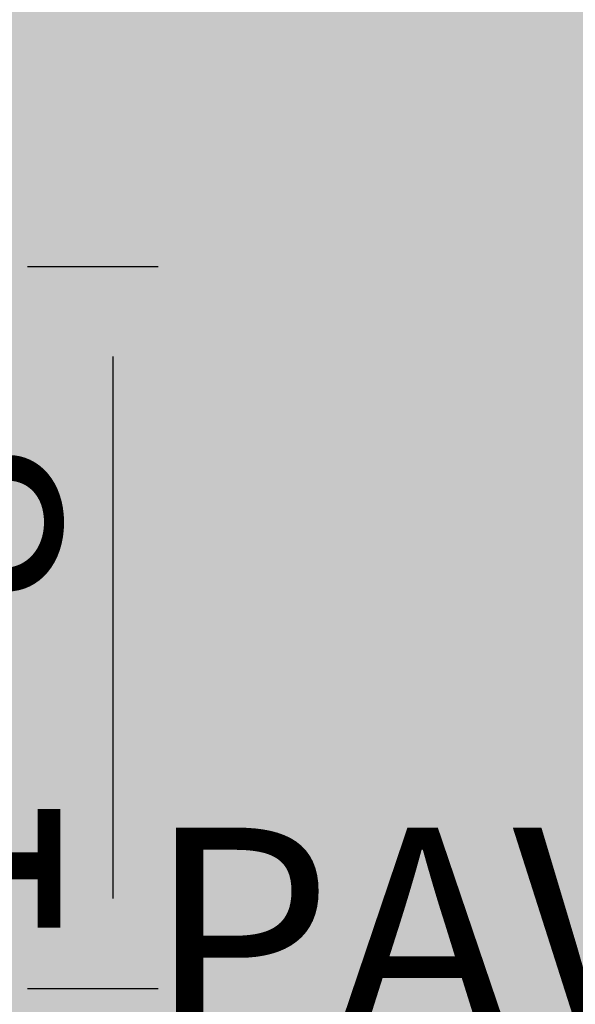
# Model space of a CAD drawing. Units: inches. Extents: x 459864 to 460310, y 324185 to 324787.
# Tile 55 of 112: x 460153 to 460169, y 324211 to 324239. Entities that reach past the tile are written whole.
import ezdxf

# ---------------------------------------------------------------- set-up
doc = ezdxf.new("R2010")
doc.units = ezdxf.units.IN
doc.layers.add('A-ANNO-DIMS', color=2, linetype='Continuous', lineweight=18)
doc.layers.add('L-SITE-PATT', color=252, linetype='Continuous', lineweight=13)
doc.styles.get("Standard").update_dxf_attribs({"font": 'arial.ttf'})
doc.dimstyles.new('ISO-25', dxfattribs={"dimtxt": 6, "dimasz": 2.5, "dimexe": 1.25, "dimexo": 0.625, "dimtad": 1, "dimdec": 1, "dimlunit": 3, "dimtxsty": 'Standard', "dimcen": 2.5, "dimadec": 0, "dimazin": 0, "dimtfac": 1, "dimtdec": 1, "dimtmove": 0, "dimatfit": 3, "dimfxl": 1, "dimarcsym": 0})

# ---------------------------------------------------------------- blocks, each defined once
blk = doc.blocks.new('*D34')
at = {"layer": 'A-ANNO-DIMS', "color": 0, "lineweight": -2, "transparency": 16777216}
for p, q in [((460132.814, 324211.063), (460132.814, 324207.434)), ((460152.838, 324211.063), (460152.838, 324207.434)), ((460135.314, 324208.684), (460150.338, 324208.684)), ((460152.838, 324208.684), (460202.984, 324208.684))]:
    blk.add_line(p, q, dxfattribs=at)
at = {"layer": 'A-ANNO-DIMS', "color": 0, "transparency": 16777216}
for points in [[(460135.314, 324209.101), (460135.314, 324208.268), (460132.814, 324208.684)], [(460150.338, 324209.101), (460150.338, 324208.268), (460152.838, 324208.684)]]:
    blk.add_solid(points, dxfattribs=at)
at = {"layer": 'Defpoints', "color": 0, "transparency": 16777216}
for p in [(460132.814, 324211.688), (460152.838, 324211.688), (460152.838, 324208.684)]:
    blk.add_point(p, dxfattribs=at)
at = {"layer": 'A-ANNO-DIMS', "color": 0, "transparency": 16777216, "insert": (460179.161, 324212.373), "char_height": 6, "attachment_point": 5}
blk.add_mtext('PAVER 1\'-8"', dxfattribs=at)
blk = doc.blocks.new('*D35')
at = {"layer": 'A-ANNO-DIMS', "color": 0, "lineweight": -2, "transparency": 16777216}
for p, q in [((460153.463, 324231.712), (460157.092, 324231.712)), ((460155.842, 324214.188), (460155.842, 324229.212)), ((460153.463, 324211.688), (460157.092, 324211.688))]:
    blk.add_line(p, q, dxfattribs=at)
at = {"layer": 'A-ANNO-DIMS', "color": 0, "transparency": 16777216}
for points in [[(460155.425, 324229.212), (460156.258, 324229.212), (460155.842, 324231.712)], [(460155.425, 324214.188), (460156.258, 324214.188), (460155.842, 324211.688)]]:
    blk.add_solid(points, dxfattribs=at)
at = {"layer": 'Defpoints', "color": 0, "transparency": 16777216}
for p in [(460152.838, 324231.712), (460155.842, 324231.712), (460152.838, 324211.688)]:
    blk.add_point(p, dxfattribs=at)
at = {"layer": 'A-ANNO-DIMS', "color": 0, "transparency": 16777216, "insert": (460152.153, 324221.7), "char_height": 6, "attachment_point": 5, "rotation": 90}
blk.add_mtext('1\'-8"', dxfattribs=at)

msp = doc.modelspace()

# ---------------------------------------------------------------- hatches: boundary and pattern name
at = {"layer": 'L-SITE-PATT'}
h = msp.add_hatch(dxfattribs=at)
h.set_pattern_fill('DOTS', color=256)
h.paths.add_polyline_path([(460269.804, 324283.483), (460247.115, 324283.483), (460121.929, 324283.483), (460121.929, 324252.473), (460117.429, 324252.473), (460110.124, 324252.473), (460110.124, 324243.287), (460080.83, 324243.287), (460080.83, 324252.473), (460061.115, 324252.473), (460061.115, 324251.882), (460077.909, 324251.882), (460077.909, 324199.483), (460080.83, 324199.483), (460080.83, 324207.553), (460110.124, 324207.553), (460110.124, 324199.483), (460110.813, 324199.483), (460262.115, 324199.483), (460269.804, 324199.483)], flags=17)
edge = h.paths.add_edge_path(flags=0)
edge.add_ellipse((460222.59, 324263.813), major_axis=(-8.485, 8.485), ratio=1, start_angle=405, end_angle=495, ccw=False)
edge.add_line((460214.821, 324254.66), (460214.832, 324254.666))
edge.add_ellipse((460222.59, 324263.813), major_axis=(-8.485, 8.485), ratio=1, start_angle=405, end_angle=495, ccw=False)
edge.add_line((460210.759, 324261.781), (460210.768, 324261.787))
edge.add_ellipse((460222.59, 324263.813), major_axis=(-8.485, 8.485), ratio=1, start_angle=405, end_angle=495, ccw=False)
edge.add_ellipse((460222.59, 324263.813), major_axis=(-8.485, 8.485), ratio=1, start_angle=392.754, end_angle=405, ccw=False)
edge.add_ellipse((460222.59, 324263.813), major_axis=(-8.485, 8.485), ratio=1, start_angle=380.9347, end_angle=392.754, ccw=False)
edge.add_line((460211.337, 324267.985), (460211.34, 324267.985))
edge.add_ellipse((460222.59, 324263.813), major_axis=(-8.485, 8.485), ratio=1, start_angle=380.9347, end_angle=392.754, ccw=False)
edge.add_ellipse((460222.59, 324263.813), major_axis=(-8.485, 8.485), ratio=1, start_angle=347.9015, end_angle=380.9347, ccw=False)
edge.add_ellipse((460222.59, 324263.813), major_axis=(-8.485, 8.485), ratio=1, start_angle=327.0619, end_angle=347.9015, ccw=False)
edge.add_ellipse((460222.59, 324263.813), major_axis=(-8.485, 8.485), ratio=1, start_angle=278.3246, end_angle=327.0619, ccw=False)
edge.add_line((460225.158, 324275.536), (460225.158, 324275.535))
edge.add_ellipse((460222.59, 324263.813), major_axis=(-8.485, 8.485), ratio=1, start_angle=278.3246, end_angle=327.0619, ccw=False)
edge.add_ellipse((460222.59, 324263.813), major_axis=(-8.485, 8.485), ratio=1, start_angle=260.6436, end_angle=278.3246, ccw=False)
edge.add_ellipse((460222.59, 324263.813), major_axis=(-8.485, 8.485), ratio=1, start_angle=225, end_angle=260.6436, ccw=False)
edge.add_line((460234.509, 324265.243), (460234.501, 324265.239))
edge.add_ellipse((460222.59, 324263.813), major_axis=(-8.485, 8.485), ratio=1, start_angle=225, end_angle=260.6436, ccw=False)
edge.add_ellipse((460222.59, 324263.813), major_axis=(-8.485, 8.485), ratio=1, start_angle=495, end_angle=585, ccw=False)
edge.add_line((460234.437, 324261.861), (460234.424, 324261.858))
edge.add_ellipse((460222.59, 324263.813), major_axis=(-8.485, 8.485), ratio=1, start_angle=495, end_angle=585, ccw=False)
edge.add_line((460227.95, 324253.067), (460227.946, 324253.083))
edge.add_ellipse((460222.59, 324263.813), major_axis=(-8.485, 8.485), ratio=1, start_angle=495, end_angle=585, ccw=False)
edge.add_line((460226.223, 324252.369), (460226.211, 324252.38))
edge.add_ellipse((460222.59, 324263.813), major_axis=(-8.485, 8.485), ratio=1, start_angle=495, end_angle=585, ccw=False)
h.paths.add_polyline_path([(460219.651, 324254.347), (460218.461, 324253.545), (460218.275, 324254.789), (460219.642, 324256.542), (460219.625, 324260.848), (460216.11, 324257.333), (460214.35, 324256.978), (460215.416, 324259.356), (460212.524, 324258.496), (460213.137, 324259.93), (460218.507, 324263.813), (460222.59, 324263.813), (460222.59, 324267.807), (460218.176, 324272.212), (460219.026, 324274.639), (460222.59, 324272.811), (460222.59, 324275.423), (460223.057, 324274.825), (460222.675, 324273.492), (460225.912, 324267.135), (460219.625, 324260.848)], flags=0)
edge = h.paths.add_edge_path(flags=0)
edge.add_ellipse((460194.576, 324264.046), major_axis=(-8.485, 8.485), ratio=1, start_angle=495, end_angle=585, ccw=False)
edge.add_line((460199.936, 324253.3), (460199.932, 324253.316))
edge.add_ellipse((460194.576, 324264.046), major_axis=(-8.485, 8.485), ratio=1, start_angle=495, end_angle=585, ccw=False)
edge.add_line((460198.208, 324252.603), (460198.196, 324252.613))
edge.add_ellipse((460194.576, 324264.046), major_axis=(-8.485, 8.485), ratio=1, start_angle=495, end_angle=585, ccw=False)
edge.add_ellipse((460194.576, 324264.046), major_axis=(-8.485, 8.485), ratio=1, start_angle=405, end_angle=495, ccw=False)
edge.add_line((460186.806, 324254.893), (460186.817, 324254.899))
edge.add_ellipse((460194.576, 324264.046), major_axis=(-8.485, 8.485), ratio=1, start_angle=405, end_angle=495, ccw=False)
edge.add_line((460182.744, 324262.014), (460182.753, 324262.02))
edge.add_ellipse((460194.576, 324264.046), major_axis=(-8.485, 8.485), ratio=1, start_angle=405, end_angle=495, ccw=False)
edge.add_ellipse((460194.576, 324264.046), major_axis=(-8.485, 8.485), ratio=1, start_angle=392.754, end_angle=405, ccw=False)
edge.add_ellipse((460194.576, 324264.046), major_axis=(-8.485, 8.485), ratio=1, start_angle=380.9347, end_angle=392.754, ccw=False)
edge.add_line((460183.323, 324268.218), (460183.326, 324268.218))
edge.add_ellipse((460194.576, 324264.046), major_axis=(-8.485, 8.485), ratio=1, start_angle=380.9347, end_angle=392.754, ccw=False)
edge.add_ellipse((460194.576, 324264.046), major_axis=(-8.485, 8.485), ratio=1, start_angle=347.9015, end_angle=380.9347, ccw=False)
edge.add_ellipse((460194.576, 324264.046), major_axis=(-8.485, 8.485), ratio=1, start_angle=327.0619, end_angle=347.9015, ccw=False)
edge.add_ellipse((460194.576, 324264.046), major_axis=(-8.485, 8.485), ratio=1, start_angle=278.3246, end_angle=327.0619, ccw=False)
edge.add_line((460197.144, 324275.769), (460197.143, 324275.768))
edge.add_ellipse((460194.576, 324264.046), major_axis=(-8.485, 8.485), ratio=1, start_angle=278.3246, end_angle=327.0619, ccw=False)
edge.add_ellipse((460194.576, 324264.046), major_axis=(-8.485, 8.485), ratio=1, start_angle=260.6436, end_angle=278.3246, ccw=False)
edge.add_ellipse((460194.576, 324264.046), major_axis=(-8.485, 8.485), ratio=1, start_angle=225, end_angle=260.6436, ccw=False)
edge.add_line((460206.494, 324265.476), (460206.487, 324265.473))
edge.add_ellipse((460194.576, 324264.046), major_axis=(-8.485, 8.485), ratio=1, start_angle=225, end_angle=260.6436, ccw=False)
edge.add_ellipse((460194.576, 324264.046), major_axis=(-8.485, 8.485), ratio=1, start_angle=495, end_angle=585, ccw=False)
edge.add_line((460206.422, 324262.094), (460206.409, 324262.091))
h.paths.add_polyline_path([(460191.61, 324261.081), (460191.637, 324254.58), (460190.447, 324253.778), (460190.261, 324255.023), (460191.628, 324256.775), (460191.61, 324261.081), (460188.096, 324257.566), (460186.335, 324257.211), (460187.402, 324259.589), (460184.509, 324258.729), (460185.123, 324260.163), (460190.493, 324264.046), (460194.576, 324264.046), (460194.576, 324268.04), (460190.161, 324272.446), (460191.011, 324274.872), (460194.576, 324273.044), (460194.576, 324275.657), (460195.043, 324275.058), (460194.661, 324273.725), (460197.897, 324267.368)], flags=0)
edge = h.paths.add_edge_path(flags=0)
edge.add_ellipse((460252.912, 324263.578), major_axis=(-8.485, 8.485), ratio=1, start_angle=405, end_angle=495, ccw=False)
edge.add_line((460241.081, 324261.545), (460241.089, 324261.551))
edge.add_ellipse((460252.912, 324263.578), major_axis=(-8.485, 8.485), ratio=1, start_angle=405, end_angle=495, ccw=False)
edge.add_ellipse((460252.912, 324263.578), major_axis=(-8.485, 8.485), ratio=1, start_angle=392.754, end_angle=405, ccw=False)
edge.add_ellipse((460252.912, 324263.578), major_axis=(-8.485, 8.485), ratio=1, start_angle=380.9347, end_angle=392.754, ccw=False)
edge.add_line((460241.659, 324267.749), (460241.662, 324267.749))
edge.add_ellipse((460252.912, 324263.578), major_axis=(-8.485, 8.485), ratio=1, start_angle=380.9347, end_angle=392.754, ccw=False)
edge.add_ellipse((460252.912, 324263.578), major_axis=(-8.485, 8.485), ratio=1, start_angle=347.9015, end_angle=380.9347, ccw=False)
edge.add_ellipse((460252.912, 324263.578), major_axis=(-8.485, 8.485), ratio=1, start_angle=327.0619, end_angle=347.9015, ccw=False)
edge.add_ellipse((460252.912, 324263.578), major_axis=(-8.485, 8.485), ratio=1, start_angle=278.3246, end_angle=327.0619, ccw=False)
edge.add_line((460255.48, 324275.3), (460255.479, 324275.299))
edge.add_ellipse((460252.912, 324263.578), major_axis=(-8.485, 8.485), ratio=1, start_angle=278.3246, end_angle=327.0619, ccw=False)
edge.add_ellipse((460252.912, 324263.578), major_axis=(-8.485, 8.485), ratio=1, start_angle=260.6436, end_angle=278.3246, ccw=False)
edge.add_ellipse((460252.912, 324263.578), major_axis=(-8.485, 8.485), ratio=1, start_angle=225, end_angle=260.6436, ccw=False)
edge.add_line((460264.83, 324265.007), (460264.823, 324265.004))
edge.add_ellipse((460252.912, 324263.578), major_axis=(-8.485, 8.485), ratio=1, start_angle=225, end_angle=260.6436, ccw=False)
edge.add_ellipse((460252.912, 324263.578), major_axis=(-8.485, 8.485), ratio=1, start_angle=495, end_angle=585, ccw=False)
edge.add_line((460264.758, 324261.626), (460264.745, 324261.622))
edge.add_ellipse((460252.912, 324263.578), major_axis=(-8.485, 8.485), ratio=1, start_angle=495, end_angle=585, ccw=False)
edge.add_line((460258.272, 324252.832), (460258.268, 324252.848))
edge.add_ellipse((460252.912, 324263.578), major_axis=(-8.485, 8.485), ratio=1, start_angle=495, end_angle=585, ccw=False)
edge.add_line((460256.545, 324252.134), (460256.533, 324252.144))
edge.add_ellipse((460252.912, 324263.578), major_axis=(-8.485, 8.485), ratio=1, start_angle=495, end_angle=585, ccw=False)
edge.add_ellipse((460252.912, 324263.578), major_axis=(-8.485, 8.485), ratio=1, start_angle=405, end_angle=495, ccw=False)
edge.add_line((460245.143, 324254.424), (460245.153, 324254.43))
h.paths.add_polyline_path([(460244.672, 324256.742), (460245.738, 324259.12), (460242.846, 324258.26), (460243.459, 324259.694), (460248.829, 324263.578), (460252.912, 324263.578), (460252.912, 324267.571), (460248.497, 324271.977), (460249.348, 324274.403), (460252.912, 324272.576), (460252.912, 324275.188), (460253.379, 324274.589), (460252.997, 324273.257), (460256.233, 324266.899), (460249.946, 324260.612), (460249.973, 324254.111), (460248.783, 324253.309), (460248.597, 324254.554), (460249.964, 324256.306), (460249.946, 324260.612), (460246.432, 324257.097)], flags=0)
edge = h.paths.add_edge_path(flags=0)
edge.add_ellipse((460167.439, 324262.833), major_axis=(-8.485, 8.485), ratio=1, start_angle=495, end_angle=585, ccw=False)
edge.add_line((460172.799, 324252.087), (460172.795, 324252.103))
edge.add_ellipse((460167.439, 324262.833), major_axis=(-8.485, 8.485), ratio=1, start_angle=495, end_angle=585, ccw=False)
edge.add_line((460171.071, 324251.389), (460171.059, 324251.399))
edge.add_ellipse((460167.439, 324262.833), major_axis=(-8.485, 8.485), ratio=1, start_angle=495, end_angle=585, ccw=False)
edge.add_ellipse((460167.439, 324262.833), major_axis=(-8.485, 8.485), ratio=1, start_angle=405, end_angle=495, ccw=False)
edge.add_line((460159.669, 324253.679), (460159.68, 324253.685))
edge.add_ellipse((460167.439, 324262.833), major_axis=(-8.485, 8.485), ratio=1, start_angle=405, end_angle=495, ccw=False)
edge.add_line((460155.607, 324260.8), (460155.616, 324260.806))
edge.add_ellipse((460167.439, 324262.833), major_axis=(-8.485, 8.485), ratio=1, start_angle=405, end_angle=495, ccw=False)
edge.add_ellipse((460167.439, 324262.833), major_axis=(-8.485, 8.485), ratio=1, start_angle=392.754, end_angle=405, ccw=False)
edge.add_ellipse((460167.439, 324262.833), major_axis=(-8.485, 8.485), ratio=1, start_angle=380.9347, end_angle=392.754, ccw=False)
edge.add_line((460156.185, 324267.005), (460156.189, 324267.005))
edge.add_ellipse((460167.439, 324262.833), major_axis=(-8.485, 8.485), ratio=1, start_angle=380.9347, end_angle=392.754, ccw=False)
edge.add_ellipse((460167.439, 324262.833), major_axis=(-8.485, 8.485), ratio=1, start_angle=347.9015, end_angle=380.9347, ccw=False)
edge.add_ellipse((460167.439, 324262.833), major_axis=(-8.485, 8.485), ratio=1, start_angle=327.0619, end_angle=347.9015, ccw=False)
edge.add_ellipse((460167.439, 324262.833), major_axis=(-8.485, 8.485), ratio=1, start_angle=278.3246, end_angle=327.0619, ccw=False)
edge.add_line((460170.007, 324274.556), (460170.006, 324274.554))
edge.add_ellipse((460167.439, 324262.833), major_axis=(-8.485, 8.485), ratio=1, start_angle=278.3246, end_angle=327.0619, ccw=False)
edge.add_ellipse((460167.439, 324262.833), major_axis=(-8.485, 8.485), ratio=1, start_angle=260.6436, end_angle=278.3246, ccw=False)
edge.add_ellipse((460167.439, 324262.833), major_axis=(-8.485, 8.485), ratio=1, start_angle=225, end_angle=260.6436, ccw=False)
edge.add_line((460179.357, 324264.262), (460179.35, 324264.259))
edge.add_ellipse((460167.439, 324262.833), major_axis=(-8.485, 8.485), ratio=1, start_angle=225, end_angle=260.6436, ccw=False)
edge.add_ellipse((460167.439, 324262.833), major_axis=(-8.485, 8.485), ratio=1, start_angle=495, end_angle=585, ccw=False)
edge.add_line((460179.285, 324260.881), (460179.272, 324260.877))
h.paths.add_polyline_path([(460164.473, 324259.867), (460164.5, 324253.366), (460163.31, 324252.565), (460163.124, 324253.809), (460164.491, 324255.561), (460164.473, 324259.867), (460160.958, 324256.353), (460159.198, 324255.998), (460160.265, 324258.375), (460157.372, 324257.515), (460157.986, 324258.949), (460163.356, 324262.833), (460167.439, 324262.833), (460167.439, 324266.826), (460163.024, 324271.232), (460163.874, 324273.659), (460167.439, 324271.831), (460167.439, 324274.443), (460167.905, 324273.844), (460167.524, 324272.512), (460170.76, 324266.154)], flags=0)
edge = h.paths.add_edge_path(flags=0)
edge.add_ellipse((460140.758, 324262.37), major_axis=(-8.485, 8.485), ratio=1, start_angle=495, end_angle=585, ccw=False)
edge.add_line((460146.118, 324251.624), (460146.114, 324251.639))
edge.add_ellipse((460140.758, 324262.37), major_axis=(-8.485, 8.485), ratio=1, start_angle=495, end_angle=585, ccw=False)
edge.add_line((460144.391, 324250.926), (460144.379, 324250.936))
edge.add_ellipse((460140.758, 324262.37), major_axis=(-8.485, 8.485), ratio=1, start_angle=495, end_angle=585, ccw=False)
edge.add_ellipse((460140.758, 324262.37), major_axis=(-8.485, 8.485), ratio=1, start_angle=405, end_angle=495, ccw=False)
edge.add_line((460132.989, 324253.216), (460132.999, 324253.222))
edge.add_ellipse((460140.758, 324262.37), major_axis=(-8.485, 8.485), ratio=1, start_angle=405, end_angle=495, ccw=False)
edge.add_line((460128.927, 324260.337), (460128.935, 324260.343))
edge.add_ellipse((460140.758, 324262.37), major_axis=(-8.485, 8.485), ratio=1, start_angle=405, end_angle=495, ccw=False)
edge.add_ellipse((460140.758, 324262.37), major_axis=(-8.485, 8.485), ratio=1, start_angle=392.754, end_angle=405, ccw=False)
edge.add_ellipse((460140.758, 324262.37), major_axis=(-8.485, 8.485), ratio=1, start_angle=380.9347, end_angle=392.754, ccw=False)
edge.add_line((460129.505, 324266.541), (460129.508, 324266.541))
edge.add_ellipse((460140.758, 324262.37), major_axis=(-8.485, 8.485), ratio=1, start_angle=380.9347, end_angle=392.754, ccw=False)
edge.add_ellipse((460140.758, 324262.37), major_axis=(-8.485, 8.485), ratio=1, start_angle=347.9015, end_angle=380.9347, ccw=False)
edge.add_ellipse((460140.758, 324262.37), major_axis=(-8.485, 8.485), ratio=1, start_angle=327.0619, end_angle=347.9015, ccw=False)
edge.add_ellipse((460140.758, 324262.37), major_axis=(-8.485, 8.485), ratio=1, start_angle=278.3246, end_angle=327.0619, ccw=False)
edge.add_line((460143.326, 324274.092), (460143.325, 324274.091))
edge.add_ellipse((460140.758, 324262.37), major_axis=(-8.485, 8.485), ratio=1, start_angle=278.3246, end_angle=327.0619, ccw=False)
edge.add_ellipse((460140.758, 324262.37), major_axis=(-8.485, 8.485), ratio=1, start_angle=260.6436, end_angle=278.3246, ccw=False)
edge.add_ellipse((460140.758, 324262.37), major_axis=(-8.485, 8.485), ratio=1, start_angle=225, end_angle=260.6436, ccw=False)
edge.add_line((460152.677, 324263.799), (460152.669, 324263.796))
edge.add_ellipse((460140.758, 324262.37), major_axis=(-8.485, 8.485), ratio=1, start_angle=225, end_angle=260.6436, ccw=False)
edge.add_ellipse((460140.758, 324262.37), major_axis=(-8.485, 8.485), ratio=1, start_angle=495, end_angle=585, ccw=False)
edge.add_line((460152.604, 324260.418), (460152.592, 324260.414))
h.paths.add_polyline_path([(460137.792, 324259.404), (460137.819, 324252.903), (460136.629, 324252.101), (460136.443, 324253.346), (460137.81, 324255.098), (460137.792, 324259.404), (460134.278, 324255.889), (460132.518, 324255.534), (460133.584, 324257.912), (460130.692, 324257.052), (460131.305, 324258.486), (460136.675, 324262.37), (460140.758, 324262.37), (460140.758, 324266.363), (460136.343, 324270.769), (460137.194, 324273.195), (460140.758, 324271.367), (460140.758, 324273.98), (460141.225, 324273.381), (460140.843, 324272.049), (460144.079, 324265.691)], flags=0)
h.paths.add_polyline_path([(460110.124, 324227.414), (460080.83, 324227.414), (460080.83, 324235.484), (460110.124, 324235.484)], flags=16)
h.paths.add_polyline_path([(460110.124, 324220.797), (460110.124, 324212.727), (460080.83, 324212.727), (460080.83, 324220.797)], flags=16)
h.paths.add_polyline_path([(460269.804, 324283.483), (460247.115, 324283.483), (460121.929, 324283.483), (460121.929, 324252.473), (460117.429, 324252.473), (460110.124, 324252.473), (460110.124, 324243.287), (460080.83, 324243.287), (460080.83, 324252.473), (460061.115, 324252.473), (460061.115, 324251.882), (460077.909, 324251.882), (460077.909, 324199.483), (460080.83, 324199.483), (460080.83, 324207.553), (460110.124, 324207.553), (460110.124, 324199.483), (460262.115, 324199.483), (460269.804, 324199.483)], flags=17)
h.paths.add_polyline_path([(460219.651, 324254.347), (460218.461, 324253.545), (460218.275, 324254.789), (460219.642, 324256.542), (460219.625, 324260.848), (460216.11, 324257.333), (460214.35, 324256.978), (460215.416, 324259.356), (460212.524, 324258.496), (460213.137, 324259.93), (460218.507, 324263.813), (460222.59, 324263.813), (460220.18, 324266.223), (460215.461, 324265.308), (460211.835, 324266.137), (460216.247, 324267.985), (460218.418, 324267.985), (460222.59, 324263.813), (460222.59, 324267.807), (460218.176, 324272.212), (460219.026, 324274.639), (460222.59, 324272.811), (460222.59, 324275.423), (460223.057, 324274.825), (460222.675, 324273.492), (460225.912, 324267.135), (460222.59, 324263.813), (460231.383, 324263.813), (460228.485, 324262.488), (460224.425, 324261.978), (460228.68, 324257.724), (460228.966, 324254.791), (460227.142, 324256.537), (460227.542, 324254.819), (460227.333, 324253.614), (460222.59, 324259.985), (460222.59, 324255.497), (460221.377, 324256.541), (460220.576, 324261.799), (460219.625, 324260.848)], flags=0)
h.paths.add_polyline_path([(460199.127, 324256.77), (460199.528, 324255.052), (460199.319, 324253.848), (460194.576, 324260.218), (460194.576, 324255.73), (460193.363, 324256.774), (460192.561, 324262.032), (460191.61, 324261.081), (460191.637, 324254.58), (460190.447, 324253.778), (460190.261, 324255.023), (460191.628, 324256.775), (460191.61, 324261.081), (460188.096, 324257.566), (460186.335, 324257.211), (460187.402, 324259.589), (460184.509, 324258.729), (460185.123, 324260.163), (460190.493, 324264.046), (460194.576, 324264.046), (460192.166, 324266.456), (460187.446, 324265.541), (460183.82, 324266.37), (460188.232, 324268.218), (460190.404, 324268.218), (460194.576, 324264.046), (460194.576, 324268.04), (460190.161, 324272.446), (460191.011, 324274.872), (460194.576, 324273.044), (460194.576, 324275.657), (460195.043, 324275.058), (460194.661, 324273.725), (460197.897, 324267.368), (460194.576, 324264.046), (460203.368, 324264.046), (460200.47, 324262.721), (460196.411, 324262.212), (460200.665, 324257.957), (460200.951, 324255.024)], flags=0)
h.paths.add_polyline_path([(460244.672, 324256.742), (460245.738, 324259.12), (460242.846, 324258.26), (460243.459, 324259.694), (460248.829, 324263.578), (460252.912, 324263.578), (460250.502, 324265.987), (460245.783, 324265.072), (460242.156, 324265.901), (460246.568, 324267.749), (460248.74, 324267.749), (460252.912, 324263.578), (460252.912, 324267.571), (460248.497, 324271.977), (460249.348, 324274.403), (460252.912, 324272.576), (460252.912, 324275.188), (460253.379, 324274.589), (460252.997, 324273.257), (460256.233, 324266.899), (460252.912, 324263.578), (460261.705, 324263.578), (460258.806, 324262.252), (460254.747, 324261.743), (460259.002, 324257.488), (460259.288, 324254.555), (460257.463, 324256.301), (460257.864, 324254.583), (460257.655, 324253.379), (460252.912, 324259.749), (460252.912, 324255.261), (460251.699, 324256.305), (460250.897, 324261.563), (460249.946, 324260.612), (460249.973, 324254.111), (460248.783, 324253.309), (460248.597, 324254.554), (460249.964, 324256.306), (460249.946, 324260.612), (460246.432, 324257.097)], flags=0)
h.paths.add_polyline_path([(460173.528, 324256.743), (460173.814, 324253.811), (460171.99, 324255.556), (460172.39, 324253.838), (460172.182, 324252.634), (460167.439, 324259.004), (460167.439, 324254.516), (460166.226, 324255.56), (460165.424, 324260.818), (460164.473, 324259.867), (460164.5, 324253.366), (460163.31, 324252.565), (460163.124, 324253.809), (460164.491, 324255.561), (460164.473, 324259.867), (460160.958, 324256.353), (460159.198, 324255.998), (460160.265, 324258.375), (460157.372, 324257.515), (460157.986, 324258.949), (460163.356, 324262.833), (460167.439, 324262.833), (460165.029, 324265.243), (460160.309, 324264.327), (460156.683, 324265.156), (460161.095, 324267.005), (460163.267, 324267.005), (460167.439, 324262.833), (460167.439, 324266.826), (460163.024, 324271.232), (460163.874, 324273.659), (460167.439, 324271.831), (460167.439, 324274.443), (460167.905, 324273.844), (460167.524, 324272.512), (460170.76, 324266.154), (460167.439, 324262.833), (460176.231, 324262.833), (460173.333, 324261.507), (460169.274, 324260.998)], flags=0)
h.paths.add_polyline_path([(460146.848, 324256.28), (460147.134, 324253.347), (460145.31, 324255.093), (460145.71, 324253.375), (460145.501, 324252.171), (460140.758, 324258.541), (460140.758, 324254.053), (460139.545, 324255.097), (460138.744, 324260.355), (460137.792, 324259.404), (460137.819, 324252.903), (460136.629, 324252.101), (460136.443, 324253.346), (460137.81, 324255.098), (460137.792, 324259.404), (460134.278, 324255.889), (460132.518, 324255.534), (460133.584, 324257.912), (460130.692, 324257.052), (460131.305, 324258.486), (460136.675, 324262.37), (460140.758, 324262.37), (460138.348, 324264.779), (460133.629, 324263.864), (460130.002, 324264.693), (460134.414, 324266.541), (460136.586, 324266.541), (460140.758, 324262.37), (460140.758, 324266.363), (460136.343, 324270.769), (460137.194, 324273.195), (460140.758, 324271.367), (460140.758, 324273.98), (460141.225, 324273.381), (460140.843, 324272.049), (460144.079, 324265.691), (460140.758, 324262.37), (460149.551, 324262.37), (460146.653, 324261.044), (460142.593, 324260.535)], flags=0)
edge = h.paths.add_edge_path()
edge.add_line((460269.804, 324272.549), (460260.881, 324272.549))
edge.add_ellipse((460252.912, 324263.578), major_axis=(-8.485, 8.485), ratio=1, start_angle=260.6436, end_angle=273.3846, ccw=False)
edge.add_line((460262.283, 324271.092), (460262.261, 324271.091))
edge.add_ellipse((460252.912, 324263.578), major_axis=(-8.485, 8.485), ratio=1, start_angle=260.6436, end_angle=273.3846, ccw=False)
edge.add_ellipse((460252.912, 324263.578), major_axis=(-8.485, 8.485), ratio=1, start_angle=225, end_angle=260.6436, ccw=False)
edge.add_line((460263.609, 324269.063), (460263.572, 324269.058))
edge.add_ellipse((460252.912, 324263.578), major_axis=(-8.485, 8.485), ratio=1, start_angle=225, end_angle=260.6436, ccw=False)
edge.add_line((460264.615, 324266.306), (460264.585, 324266.305))
edge.add_ellipse((460252.912, 324263.578), major_axis=(-8.485, 8.485), ratio=1, start_angle=225, end_angle=260.6436, ccw=False)
edge.add_line((460264.83, 324265.007), (460264.823, 324265.004))
edge.add_ellipse((460252.912, 324263.578), major_axis=(-8.485, 8.485), ratio=1, start_angle=225, end_angle=260.6436, ccw=False)
edge.add_ellipse((460252.912, 324263.578), major_axis=(-8.485, 8.485), ratio=1, start_angle=495, end_angle=585, ccw=False)
edge.add_line((460264.758, 324261.626), (460264.745, 324261.622))
edge.add_ellipse((460252.912, 324263.578), major_axis=(-8.485, 8.485), ratio=1, start_angle=495, end_angle=585, ccw=False)
edge.add_line((460263.442, 324257.739), (460263.389, 324257.779))
edge.add_ellipse((460252.912, 324263.578), major_axis=(-8.485, 8.485), ratio=1, start_angle=495, end_angle=585, ccw=False)
edge.add_line((460258.128, 324252.744), (460258.102, 324252.779))
edge.add_ellipse((460252.912, 324263.578), major_axis=(-8.485, 8.485), ratio=1, start_angle=495, end_angle=585, ccw=False)
edge.add_line((460256.545, 324252.134), (460256.533, 324252.144))
edge.add_ellipse((460252.912, 324263.578), major_axis=(-8.485, 8.485), ratio=1, start_angle=495, end_angle=585, ccw=False)
edge.add_ellipse((460252.912, 324263.578), major_axis=(-8.485, 8.485), ratio=1, start_angle=405, end_angle=495, ccw=False)
edge.add_line((460250.594, 324251.78), (460250.605, 324251.82))
edge.add_ellipse((460252.912, 324263.578), major_axis=(-8.485, 8.485), ratio=1, start_angle=405, end_angle=495, ccw=False)
edge.add_line((460245.143, 324254.424), (460245.153, 324254.43))
edge.add_ellipse((460252.912, 324263.578), major_axis=(-8.485, 8.485), ratio=1, start_angle=405, end_angle=495, ccw=False)
edge.add_line((460243.525, 324256.059), (460243.56, 324256.091))
edge.add_ellipse((460252.912, 324263.578), major_axis=(-8.485, 8.485), ratio=1, start_angle=405, end_angle=495, ccw=False)
edge.add_line((460241.44, 324259.893), (460241.522, 324259.896))
edge.add_ellipse((460252.912, 324263.578), major_axis=(-8.485, 8.485), ratio=1, start_angle=405, end_angle=495, ccw=False)
edge.add_line((460241.081, 324261.545), (460241.089, 324261.551))
edge.add_ellipse((460252.912, 324263.578), major_axis=(-8.485, 8.485), ratio=1, start_angle=405, end_angle=495, ccw=False)
edge.add_ellipse((460252.912, 324263.578), major_axis=(-8.485, 8.485), ratio=1, start_angle=392.754, end_angle=405, ccw=False)
edge.add_line((460241.05, 324265.438), (460241.063, 324265.443))
edge.add_ellipse((460252.912, 324263.578), major_axis=(-8.485, 8.485), ratio=1, start_angle=392.754, end_angle=405, ccw=False)
edge.add_ellipse((460252.912, 324263.578), major_axis=(-8.485, 8.485), ratio=1, start_angle=380.9347, end_angle=392.754, ccw=False)
edge.add_line((460241.452, 324267.176), (460241.469, 324267.171))
edge.add_ellipse((460252.912, 324263.578), major_axis=(-8.485, 8.485), ratio=1, start_angle=380.9347, end_angle=392.754, ccw=False)
edge.add_line((460241.659, 324267.749), (460241.662, 324267.749))
edge.add_ellipse((460252.912, 324263.578), major_axis=(-8.485, 8.485), ratio=1, start_angle=380.9347, end_angle=392.754, ccw=False)
edge.add_ellipse((460252.912, 324263.578), major_axis=(-8.485, 8.485), ratio=1, start_angle=356.6154, end_angle=380.9347, ccw=False)
edge.add_line((460244.88, 324272.488), (460244.713, 324272.549))
edge.add_line((460244.713, 324272.549), (460230.817, 324272.549))
edge.add_ellipse((460222.59, 324263.813), major_axis=(-8.485, 8.485), ratio=1, start_angle=260.6436, end_angle=271.7178, ccw=False)
edge.add_ellipse((460222.59, 324263.813), major_axis=(-8.485, 8.485), ratio=1, start_angle=225, end_angle=260.6436, ccw=False)
edge.add_line((460233.287, 324269.299), (460233.25, 324269.294))
edge.add_ellipse((460222.59, 324263.813), major_axis=(-8.485, 8.485), ratio=1, start_angle=225, end_angle=260.6436, ccw=False)
edge.add_line((460234.294, 324266.541), (460234.264, 324266.541))
edge.add_ellipse((460222.59, 324263.813), major_axis=(-8.485, 8.485), ratio=1, start_angle=225, end_angle=260.6436, ccw=False)
edge.add_line((460234.509, 324265.243), (460234.501, 324265.239))
edge.add_ellipse((460222.59, 324263.813), major_axis=(-8.485, 8.485), ratio=1, start_angle=225, end_angle=260.6436, ccw=False)
edge.add_ellipse((460222.59, 324263.813), major_axis=(-8.485, 8.485), ratio=1, start_angle=495, end_angle=585, ccw=False)
edge.add_line((460234.437, 324261.861), (460234.424, 324261.858))
edge.add_ellipse((460222.59, 324263.813), major_axis=(-8.485, 8.485), ratio=1, start_angle=495, end_angle=585, ccw=False)
edge.add_line((460233.121, 324257.975), (460233.068, 324258.015))
edge.add_ellipse((460222.59, 324263.813), major_axis=(-8.485, 8.485), ratio=1, start_angle=495, end_angle=585, ccw=False)
edge.add_line((460227.806, 324252.979), (460227.78, 324253.014))
edge.add_ellipse((460222.59, 324263.813), major_axis=(-8.485, 8.485), ratio=1, start_angle=495, end_angle=585, ccw=False)
edge.add_line((460226.223, 324252.369), (460226.211, 324252.38))
edge.add_ellipse((460222.59, 324263.813), major_axis=(-8.485, 8.485), ratio=1, start_angle=495, end_angle=585, ccw=False)
edge.add_ellipse((460222.59, 324263.813), major_axis=(-8.485, 8.485), ratio=1, start_angle=405, end_angle=495, ccw=False)
edge.add_line((460220.272, 324252.016), (460220.283, 324252.055))
edge.add_ellipse((460222.59, 324263.813), major_axis=(-8.485, 8.485), ratio=1, start_angle=405, end_angle=495, ccw=False)
edge.add_line((460214.821, 324254.66), (460214.832, 324254.666))
edge.add_ellipse((460222.59, 324263.813), major_axis=(-8.485, 8.485), ratio=1, start_angle=405, end_angle=495, ccw=False)
edge.add_line((460213.203, 324256.295), (460213.239, 324256.327))
edge.add_ellipse((460222.59, 324263.813), major_axis=(-8.485, 8.485), ratio=1, start_angle=405, end_angle=495, ccw=False)
edge.add_line((460211.118, 324260.128), (460211.201, 324260.131))
edge.add_ellipse((460222.59, 324263.813), major_axis=(-8.485, 8.485), ratio=1, start_angle=405, end_angle=495, ccw=False)
edge.add_line((460210.759, 324261.781), (460210.768, 324261.787))
edge.add_ellipse((460222.59, 324263.813), major_axis=(-8.485, 8.485), ratio=1, start_angle=405, end_angle=495, ccw=False)
edge.add_ellipse((460222.59, 324263.813), major_axis=(-8.485, 8.485), ratio=1, start_angle=392.754, end_angle=405, ccw=False)
edge.add_line((460210.729, 324265.673), (460210.741, 324265.678))
edge.add_ellipse((460222.59, 324263.813), major_axis=(-8.485, 8.485), ratio=1, start_angle=392.754, end_angle=405, ccw=False)
edge.add_ellipse((460222.59, 324263.813), major_axis=(-8.485, 8.485), ratio=1, start_angle=380.9347, end_angle=392.754, ccw=False)
edge.add_line((460211.13, 324267.412), (460211.147, 324267.407))
edge.add_ellipse((460222.59, 324263.813), major_axis=(-8.485, 8.485), ratio=1, start_angle=380.9347, end_angle=392.754, ccw=False)
edge.add_line((460211.337, 324267.985), (460211.34, 324267.985))
edge.add_ellipse((460222.59, 324263.813), major_axis=(-8.485, 8.485), ratio=1, start_angle=380.9347, end_angle=392.754, ccw=False)
edge.add_ellipse((460222.59, 324263.813), major_axis=(-8.485, 8.485), ratio=1, start_angle=358.2822, end_angle=380.9347, ccw=False)
edge.add_line((460213.705, 324271.902), (460213.709, 324271.869))
edge.add_ellipse((460222.59, 324263.813), major_axis=(-8.485, 8.485), ratio=1, start_angle=358.2822, end_angle=380.9347, ccw=False)
edge.add_line((460214.363, 324272.549), (460203.078, 324272.549))
edge.add_line((460203.078, 324272.549), (460203.06, 324272.531))
edge.add_ellipse((460194.576, 324264.046), major_axis=(-8.485, 8.485), ratio=1, start_angle=260.6436, end_angle=270.1168, ccw=False)
edge.add_line((460203.957, 324271.561), (460203.921, 324271.56))
edge.add_ellipse((460194.576, 324264.046), major_axis=(-8.485, 8.485), ratio=1, start_angle=260.6436, end_angle=270.1168, ccw=False)
edge.add_ellipse((460194.576, 324264.046), major_axis=(-8.485, 8.485), ratio=1, start_angle=225, end_angle=260.6436, ccw=False)
edge.add_line((460205.272, 324269.532), (460205.235, 324269.527))
edge.add_ellipse((460194.576, 324264.046), major_axis=(-8.485, 8.485), ratio=1, start_angle=225, end_angle=260.6436, ccw=False)
edge.add_line((460206.279, 324266.774), (460206.249, 324266.774))
edge.add_ellipse((460194.576, 324264.046), major_axis=(-8.485, 8.485), ratio=1, start_angle=225, end_angle=260.6436, ccw=False)
edge.add_line((460206.494, 324265.476), (460206.487, 324265.473))
edge.add_ellipse((460194.576, 324264.046), major_axis=(-8.485, 8.485), ratio=1, start_angle=225, end_angle=260.6436, ccw=False)
edge.add_ellipse((460194.576, 324264.046), major_axis=(-8.485, 8.485), ratio=1, start_angle=495, end_angle=585, ccw=False)
edge.add_line((460206.422, 324262.094), (460206.409, 324262.091))
edge.add_ellipse((460194.576, 324264.046), major_axis=(-8.485, 8.485), ratio=1, start_angle=495, end_angle=585, ccw=False)
edge.add_line((460205.106, 324258.208), (460205.053, 324258.248))
edge.add_ellipse((460194.576, 324264.046), major_axis=(-8.485, 8.485), ratio=1, start_angle=495, end_angle=585, ccw=False)
edge.add_line((460199.792, 324253.212), (460199.766, 324253.248))
edge.add_ellipse((460194.576, 324264.046), major_axis=(-8.485, 8.485), ratio=1, start_angle=495, end_angle=585, ccw=False)
edge.add_line((460198.208, 324252.603), (460198.196, 324252.613))
edge.add_ellipse((460194.576, 324264.046), major_axis=(-8.485, 8.485), ratio=1, start_angle=495, end_angle=585, ccw=False)
edge.add_ellipse((460194.576, 324264.046), major_axis=(-8.485, 8.485), ratio=1, start_angle=405, end_angle=495, ccw=False)
edge.add_line((460192.258, 324252.249), (460192.268, 324252.289))
edge.add_ellipse((460194.576, 324264.046), major_axis=(-8.485, 8.485), ratio=1, start_angle=405, end_angle=495, ccw=False)
edge.add_line((460186.806, 324254.893), (460186.817, 324254.899))
edge.add_ellipse((460194.576, 324264.046), major_axis=(-8.485, 8.485), ratio=1, start_angle=405, end_angle=495, ccw=False)
edge.add_line((460185.188, 324256.528), (460185.224, 324256.56))
edge.add_ellipse((460194.576, 324264.046), major_axis=(-8.485, 8.485), ratio=1, start_angle=405, end_angle=495, ccw=False)
edge.add_line((460183.104, 324260.362), (460183.186, 324260.365))
edge.add_ellipse((460194.576, 324264.046), major_axis=(-8.485, 8.485), ratio=1, start_angle=405, end_angle=495, ccw=False)
edge.add_line((460182.744, 324262.014), (460182.753, 324262.02))
edge.add_ellipse((460194.576, 324264.046), major_axis=(-8.485, 8.485), ratio=1, start_angle=405, end_angle=495, ccw=False)
edge.add_ellipse((460194.576, 324264.046), major_axis=(-8.485, 8.485), ratio=1, start_angle=392.754, end_angle=405, ccw=False)
edge.add_line((460182.714, 324265.906), (460182.726, 324265.912))
edge.add_ellipse((460194.576, 324264.046), major_axis=(-8.485, 8.485), ratio=1, start_angle=392.754, end_angle=405, ccw=False)
edge.add_ellipse((460194.576, 324264.046), major_axis=(-8.485, 8.485), ratio=1, start_angle=380.9347, end_angle=392.754, ccw=False)
edge.add_line((460183.116, 324267.645), (460183.133, 324267.64))
edge.add_ellipse((460194.576, 324264.046), major_axis=(-8.485, 8.485), ratio=1, start_angle=380.9347, end_angle=392.754, ccw=False)
edge.add_line((460183.323, 324268.218), (460183.326, 324268.218))
edge.add_ellipse((460194.576, 324264.046), major_axis=(-8.485, 8.485), ratio=1, start_angle=380.9347, end_angle=392.754, ccw=False)
edge.add_ellipse((460194.576, 324264.046), major_axis=(-8.485, 8.485), ratio=1, start_angle=359.8832, end_angle=380.9347, ccw=False)
edge.add_line((460184.491, 324270.611), (460184.553, 324270.611))
edge.add_ellipse((460194.576, 324264.046), major_axis=(-8.485, 8.485), ratio=1, start_angle=359.8832, end_angle=380.9347, ccw=False)
edge.add_line((460185.346, 324271.76), (460185.379, 324271.728))
edge.add_ellipse((460194.576, 324264.046), major_axis=(-8.485, 8.485), ratio=1, start_angle=359.8832, end_angle=380.9347, ccw=False)
edge.add_line((460185.697, 324272.086), (460185.633, 324272.549))
edge.add_line((460185.633, 324272.549), (460174.683, 324272.549))
edge.add_line((460174.683, 324272.549), (460174.606, 324272.457))
edge.add_ellipse((460167.439, 324262.833), major_axis=(-8.485, 8.485), ratio=1, start_angle=260.6436, end_angle=278.3246, ccw=False)
edge.add_ellipse((460167.439, 324262.833), major_axis=(-8.485, 8.485), ratio=1, start_angle=225, end_angle=260.6436, ccw=False)
edge.add_line((460178.135, 324268.318), (460178.098, 324268.313))
edge.add_ellipse((460167.439, 324262.833), major_axis=(-8.485, 8.485), ratio=1, start_angle=225, end_angle=260.6436, ccw=False)
edge.add_line((460179.142, 324265.561), (460179.112, 324265.56))
edge.add_ellipse((460167.439, 324262.833), major_axis=(-8.485, 8.485), ratio=1, start_angle=225, end_angle=260.6436, ccw=False)
edge.add_line((460179.357, 324264.262), (460179.35, 324264.259))
edge.add_ellipse((460167.439, 324262.833), major_axis=(-8.485, 8.485), ratio=1, start_angle=225, end_angle=260.6436, ccw=False)
edge.add_ellipse((460167.439, 324262.833), major_axis=(-8.485, 8.485), ratio=1, start_angle=495, end_angle=585, ccw=False)
edge.add_line((460179.285, 324260.881), (460179.272, 324260.877))
edge.add_ellipse((460167.439, 324262.833), major_axis=(-8.485, 8.485), ratio=1, start_angle=495, end_angle=585, ccw=False)
edge.add_line((460177.969, 324256.994), (460177.916, 324257.034))
edge.add_ellipse((460167.439, 324262.833), major_axis=(-8.485, 8.485), ratio=1, start_angle=495, end_angle=585, ccw=False)
edge.add_line((460172.655, 324251.999), (460172.629, 324252.034))
edge.add_ellipse((460167.439, 324262.833), major_axis=(-8.485, 8.485), ratio=1, start_angle=495, end_angle=585, ccw=False)
edge.add_line((460171.071, 324251.389), (460171.059, 324251.399))
edge.add_ellipse((460167.439, 324262.833), major_axis=(-8.485, 8.485), ratio=1, start_angle=495, end_angle=585, ccw=False)
edge.add_ellipse((460167.439, 324262.833), major_axis=(-8.485, 8.485), ratio=1, start_angle=405, end_angle=495, ccw=False)
edge.add_line((460165.121, 324251.036), (460165.131, 324251.075))
edge.add_ellipse((460167.439, 324262.833), major_axis=(-8.485, 8.485), ratio=1, start_angle=405, end_angle=495, ccw=False)
edge.add_line((460159.669, 324253.679), (460159.68, 324253.685))
edge.add_ellipse((460167.439, 324262.833), major_axis=(-8.485, 8.485), ratio=1, start_angle=405, end_angle=495, ccw=False)
edge.add_line((460158.051, 324255.314), (460158.087, 324255.347))
edge.add_ellipse((460167.439, 324262.833), major_axis=(-8.485, 8.485), ratio=1, start_angle=405, end_angle=495, ccw=False)
edge.add_line((460155.967, 324259.148), (460156.049, 324259.151))
edge.add_ellipse((460167.439, 324262.833), major_axis=(-8.485, 8.485), ratio=1, start_angle=405, end_angle=495, ccw=False)
edge.add_line((460155.607, 324260.8), (460155.616, 324260.806))
edge.add_ellipse((460167.439, 324262.833), major_axis=(-8.485, 8.485), ratio=1, start_angle=405, end_angle=495, ccw=False)
edge.add_ellipse((460167.439, 324262.833), major_axis=(-8.485, 8.485), ratio=1, start_angle=392.754, end_angle=405, ccw=False)
edge.add_line((460155.577, 324264.693), (460155.589, 324264.698))
edge.add_ellipse((460167.439, 324262.833), major_axis=(-8.485, 8.485), ratio=1, start_angle=392.754, end_angle=405, ccw=False)
edge.add_ellipse((460167.439, 324262.833), major_axis=(-8.485, 8.485), ratio=1, start_angle=380.9347, end_angle=392.754, ccw=False)
edge.add_line((460155.979, 324266.432), (460155.996, 324266.426))
edge.add_ellipse((460167.439, 324262.833), major_axis=(-8.485, 8.485), ratio=1, start_angle=380.9347, end_angle=392.754, ccw=False)
edge.add_line((460156.185, 324267.005), (460156.189, 324267.005))
edge.add_ellipse((460167.439, 324262.833), major_axis=(-8.485, 8.485), ratio=1, start_angle=380.9347, end_angle=392.754, ccw=False)
edge.add_ellipse((460167.439, 324262.833), major_axis=(-8.485, 8.485), ratio=1, start_angle=350.9345, end_angle=380.9347, ccw=False)
edge.add_line((460157.363, 324269.397), (460157.414, 324269.397))
edge.add_ellipse((460167.439, 324262.833), major_axis=(-8.485, 8.485), ratio=1, start_angle=350.9345, end_angle=380.9347, ccw=False)
edge.add_line((460158.221, 324270.535), (460158.236, 324270.519))
edge.add_ellipse((460167.439, 324262.833), major_axis=(-8.485, 8.485), ratio=1, start_angle=350.9345, end_angle=380.9347, ccw=False)
edge.add_line((460159.379, 324271.753), (460159.419, 324271.738))
edge.add_ellipse((460167.439, 324262.833), major_axis=(-8.485, 8.485), ratio=1, start_angle=350.9345, end_angle=380.9347, ccw=False)
edge.add_line((460160.396, 324272.549), (460147.112, 324272.549))
edge.add_ellipse((460140.758, 324262.37), major_axis=(-8.485, 8.485), ratio=1, start_angle=278.3246, end_angle=283.0261, ccw=False)
edge.add_ellipse((460140.758, 324262.37), major_axis=(-8.485, 8.485), ratio=1, start_angle=260.6436, end_angle=278.3246, ccw=False)
edge.add_ellipse((460140.758, 324262.37), major_axis=(-8.485, 8.485), ratio=1, start_angle=225, end_angle=260.6436, ccw=False)
edge.add_line((460151.455, 324267.855), (460151.418, 324267.85))
edge.add_ellipse((460140.758, 324262.37), major_axis=(-8.485, 8.485), ratio=1, start_angle=225, end_angle=260.6436, ccw=False)
edge.add_line((460152.462, 324265.098), (460152.431, 324265.097))
edge.add_ellipse((460140.758, 324262.37), major_axis=(-8.485, 8.485), ratio=1, start_angle=225, end_angle=260.6436, ccw=False)
edge.add_line((460152.677, 324263.799), (460152.669, 324263.796))
edge.add_ellipse((460140.758, 324262.37), major_axis=(-8.485, 8.485), ratio=1, start_angle=225, end_angle=260.6436, ccw=False)
edge.add_ellipse((460140.758, 324262.37), major_axis=(-8.485, 8.485), ratio=1, start_angle=495, end_angle=585, ccw=False)
edge.add_line((460152.604, 324260.418), (460152.592, 324260.414))
edge.add_ellipse((460140.758, 324262.37), major_axis=(-8.485, 8.485), ratio=1, start_angle=495, end_angle=585, ccw=False)
edge.add_line((460151.288, 324256.531), (460151.235, 324256.571))
edge.add_ellipse((460140.758, 324262.37), major_axis=(-8.485, 8.485), ratio=1, start_angle=495, end_angle=585, ccw=False)
edge.add_line((460145.974, 324251.535), (460145.948, 324251.571))
edge.add_ellipse((460140.758, 324262.37), major_axis=(-8.485, 8.485), ratio=1, start_angle=495, end_angle=585, ccw=False)
edge.add_line((460144.391, 324250.926), (460144.379, 324250.936))
edge.add_ellipse((460140.758, 324262.37), major_axis=(-8.485, 8.485), ratio=1, start_angle=495, end_angle=585, ccw=False)
edge.add_ellipse((460140.758, 324262.37), major_axis=(-8.485, 8.485), ratio=1, start_angle=405, end_angle=495, ccw=False)
edge.add_line((460138.44, 324250.572), (460138.451, 324250.612))
edge.add_ellipse((460140.758, 324262.37), major_axis=(-8.485, 8.485), ratio=1, start_angle=405, end_angle=495, ccw=False)
edge.add_line((460132.989, 324253.216), (460132.999, 324253.222))
edge.add_ellipse((460140.758, 324262.37), major_axis=(-8.485, 8.485), ratio=1, start_angle=405, end_angle=495, ccw=False)
edge.add_line((460131.371, 324254.851), (460131.406, 324254.883))
edge.add_ellipse((460140.758, 324262.37), major_axis=(-8.485, 8.485), ratio=1, start_angle=405, end_angle=495, ccw=False)
edge.add_line((460129.286, 324258.685), (460129.369, 324258.688))
edge.add_ellipse((460140.758, 324262.37), major_axis=(-8.485, 8.485), ratio=1, start_angle=405, end_angle=495, ccw=False)
edge.add_line((460128.927, 324260.337), (460128.935, 324260.343))
edge.add_ellipse((460140.758, 324262.37), major_axis=(-8.485, 8.485), ratio=1, start_angle=405, end_angle=495, ccw=False)
edge.add_ellipse((460140.758, 324262.37), major_axis=(-8.485, 8.485), ratio=1, start_angle=392.754, end_angle=405, ccw=False)
edge.add_line((460128.896, 324264.23), (460128.909, 324264.235))
edge.add_ellipse((460140.758, 324262.37), major_axis=(-8.485, 8.485), ratio=1, start_angle=392.754, end_angle=405, ccw=False)
edge.add_ellipse((460140.758, 324262.37), major_axis=(-8.485, 8.485), ratio=1, start_angle=380.9347, end_angle=392.754, ccw=False)
edge.add_line((460129.298, 324265.968), (460129.315, 324265.963))
edge.add_ellipse((460140.758, 324262.37), major_axis=(-8.485, 8.485), ratio=1, start_angle=380.9347, end_angle=392.754, ccw=False)
edge.add_line((460129.505, 324266.541), (460129.508, 324266.541))
edge.add_ellipse((460140.758, 324262.37), major_axis=(-8.485, 8.485), ratio=1, start_angle=380.9347, end_angle=392.754, ccw=False)
edge.add_ellipse((460140.758, 324262.37), major_axis=(-8.485, 8.485), ratio=1, start_angle=347.9015, end_angle=380.9347, ccw=False)
edge.add_line((460130.697, 324268.934), (460130.727, 324268.934))
edge.add_ellipse((460140.758, 324262.37), major_axis=(-8.485, 8.485), ratio=1, start_angle=347.9015, end_angle=380.9347, ccw=False)
edge.add_line((460131.869, 324270.48), (460131.879, 324270.413))
edge.add_ellipse((460140.758, 324262.37), major_axis=(-8.485, 8.485), ratio=1, start_angle=347.9015, end_angle=380.9347, ccw=False)
edge.add_line((460132.734, 324271.277), (460132.705, 324271.287))
edge.add_ellipse((460140.758, 324262.37), major_axis=(-8.485, 8.485), ratio=1, start_angle=347.9015, end_angle=380.9347, ccw=False)
edge.add_line((460134.24, 324272.445), (460134.204, 324272.549))
edge.add_line((460134.204, 324272.549), (460121.929, 324272.549))
edge.add_line((460121.929, 324272.549), (460121.929, 324252.473))
edge.add_line((460121.929, 324252.473), (460117.429, 324252.473))
edge.add_line((460117.429, 324252.473), (460110.124, 324252.473))
edge.add_line((460110.124, 324252.473), (460110.124, 324243.287))
edge.add_line((460110.124, 324243.287), (460080.83, 324243.287))
edge.add_line((460080.83, 324243.287), (460080.83, 324252.473))
edge.add_line((460080.83, 324252.473), (460061.115, 324252.473))
edge.add_line((460061.115, 324252.473), (460061.115, 324251.882))
edge.add_line((460061.115, 324251.882), (460077.909, 324251.882))
edge.add_line((460077.909, 324251.882), (460077.909, 324199.483))
edge.add_line((460077.909, 324199.483), (460080.83, 324199.483))
edge.add_line((460080.83, 324199.483), (460080.83, 324207.553))
edge.add_line((460080.83, 324207.553), (460110.124, 324207.553))
edge.add_line((460110.124, 324207.553), (460110.124, 324199.483))
edge.add_line((460110.124, 324199.483), (460110.813, 324199.483))
edge.add_line((460110.813, 324199.483), (460262.115, 324199.483))
edge.add_line((460262.115, 324199.483), (460269.804, 324199.483))
edge.add_line((460269.804, 324199.483), (460269.804, 324272.549))

# ---------------------------------------------------------------- dimensions: what is measured, and where the dimension line sits
at = {"layer": 'A-ANNO-DIMS'}
dim = msp.add_linear_dim(base=(460155.842, 324231.712), p1=(460152.838, 324211.688), p2=(460152.838, 324231.712), angle=90, dimstyle='ISO-25', override={"dimdec": 1, "dimlfac": 1, "dimrnd": 0, "dimzin": 1, "dimdsep": 46, "dimlunit": 4, "dimfrac": 2}, dxfattribs=at)
dim.commit()
dim.dimension.update_dxf_attribs({"geometry": '*D35', "text_midpoint": (460152.153, 324221.7)})
dim = msp.add_linear_dim(base=(460152.838, 324208.684), p1=(460132.814, 324211.688), p2=(460152.838, 324211.688), text='PAVER <>', dimstyle='ISO-25', override={"dimdec": 1, "dimlfac": 1, "dimrnd": 0, "dimzin": 1, "dimdsep": 46, "dimlunit": 4, "dimfrac": 2}, dxfattribs=at)
dim.commit()
dim.dimension.update_dxf_attribs({"geometry": '*D34', "text_midpoint": (460179.161, 324212.373)})

doc.saveas('drawing.dxf')
